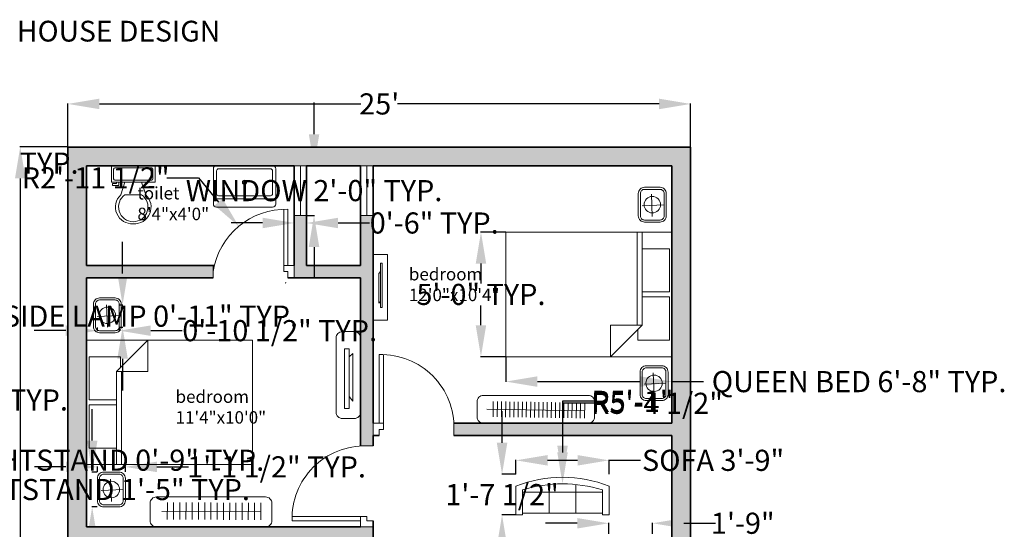
# Model space of a CAD drawing. Units: inches. Extents: x 19 to 15718, y 7 to 930.
# Tile 11 of 11: x 15243 to 15718, y 646 to 892. Entities that reach past the tile are written whole.
import ezdxf

# ---------------------------------------------------------------- set-up
doc = ezdxf.new("R2010")
doc.units = ezdxf.units.IN
doc.header["$MEASUREMENT"] = 0
for name, color, linetype, lineweight in [('A-ANNO-DIMS', 2, 'Continuous', 18), ('A-ANNO-TEXT', 7, 'Continuous', 25), ('A-AREA-IDEN', 7, 'Continuous', 18), ('A-DOOR', 4, 'Continuous', 20), ('A-FLOR-CASE', 8, 'Continuous', 18), ('A-FLOR-FIXT', 9, 'Continuous', 18), ('A-FURN', 8, 'Continuous', 18), ('A-GLAZ', 4, 'Continuous', 18), ('A-WALL', 7, 'Continuous', 35)]:
    doc.layers.add(name, color=color, linetype=linetype, lineweight=lineweight)
doc.layers.add('A-WALL-PATT', color=18, linetype='Continuous', lineweight=13, true_color=0x000000)
doc.styles.add('Annotative', font='arial.ttf')
doc.styles.get("Standard").update_dxf_attribs({"font": 'arial.ttf'})
doc.dimstyles.get("Standard").update_dxf_attribs({"dimtxt": 10.18, "dimasz": 15.18, "dimexe": 0.18, "dimexo": 0.0625, "dimgap": 0.09, "dimtad": 0, "dimtih": 1, "dimtoh": 1, "dimdec": 0, "dimzin": 0, "dimdsep": 46, "dimlunit": 3, "dimtxsty": 'Standard', "dimcen": 0.09, "dimadec": 0, "dimazin": 0, "dimtfac": 1, "dimtdec": 0, "dimtofl": 0, "dimtmove": 0, "dimatfit": 3, "dimfxl": 1, "dimtolj": 1, "dimtzin": 0, "dimarcsym": 0})

# ---------------------------------------------------------------- blocks, each defined once
blk = doc.blocks.new('Bed - Queen')
for p, q in [((0, -80.00003), (0, 0)), ((0, 0), (59.99999, 0)), ((59.99999, 0), (59.99999, -80.00003)), ((7.99999, -1.2), (28.79998, -1.2)), ((7.99999, -14.4), (7.99999, -1.2)), ((28.79998, -1.2), (28.79998, -14.4)), ((31.19999, -1.2), (51.99999, -1.2)), ((31.19999, -14.4), (31.19999, -1.2)), ((51.99999, -1.2), (51.99999, -16.4)), ((0, -14.4), (44.8, -14.4)), ((44.8, -16.8), (0, -16.8)), ((59.99999, -29.6), (44.8, -14.4)), ((44.8, -14.4), (44.8, -29.6)), ((51.99999, -16.4), (46.79936, -16.4)), ((44.8, -29.6), (59.99999, -29.6)), ((59.99999, -80.00003), (0, -80.00003))]:
    blk.add_line(p, q)
blk = doc.blocks.new('Sofa - Roundback 7 ft.')
for p, q in [((-12.00002, -32.4421), (-12.00003, -6.5971)), ((11.99997, -32.4421), (11.99998, -6.5971)), ((-36.000027, -34), (-36.000027, -11.4696)), ((-35.999844, -13.3819), (35.9998, -13.3819)), ((35.99998, -34), (35.99998, -11.4696)), ((-36.000027, -32.4421), (35.99998, -32.4421))]:
    blk.add_line(p, q)
for points in [[(-36.000027, -34), (-42.000027, -34), (-42.000027, -8)], [(41.99998, -8), (41.99998, -34), (35.99998, -34)]]:
    blk.add_lwpolyline(points)
for centre, radius, start, end in [((0, -114.25), 114.25, 68.43141, 111.5686), ((-0.00001, -127.1968), 121.1968, 72.72033, 107.2797)]:
    blk.add_arc(centre, radius, start, end)
blk = doc.blocks.new('*D16')
at = {"layer": 'A-ANNO-DIMS', "color": 0, "lineweight": -2, "transparency": 16777216}
for p, q in [((15266.68, 830.27), (15266.68, 851.13)), ((15281.86, 850.95), (15407.87, 850.95)), ((15551.5, 850.95), (15425.5, 850.95)), ((15566.68, 830.27), (15566.68, 851.13))]:
    blk.add_line(p, q, dxfattribs=at)
at = {"layer": 'A-ANNO-DIMS', "color": 0, "transparency": 16777216}
for points in [[(15281.86, 853.48), (15281.86, 848.42), (15266.68, 850.95)], [(15551.5, 853.48), (15551.5, 848.42), (15566.68, 850.95)]]:
    blk.add_solid(points, dxfattribs=at)
at = {"layer": 'Defpoints', "color": 0, "transparency": 16777216}
for p in [(15566.68, 850.95), (15266.68, 830.2), (15566.68, 830.2)]:
    blk.add_point(p, dxfattribs=at)
at = {"layer": 'A-ANNO-DIMS', "color": 0, "transparency": 16777216, "insert": (15416.68, 850.95), "char_height": 10.18, "attachment_point": 5}
blk.add_mtext("\\A1;25'", dxfattribs=at)
blk = doc.blocks.new('*D17')
at = {"layer": 'A-ANNO-DIMS', "color": 0, "lineweight": -2, "transparency": 16777216}
for p, q in [((15266.62, 830.27), (15243.58, 830.27)), ((15243.76, 815.09), (15243.76, 595.52)), ((15243.76, 365.38), (15243.76, 584.95)), ((15266.62, 350.2), (15243.58, 350.2))]:
    blk.add_line(p, q, dxfattribs=at)
at = {"layer": 'A-ANNO-DIMS', "color": 0, "transparency": 16777216}
for points in [[(15241.23, 815.09), (15246.29, 815.09), (15243.76, 830.27)], [(15241.23, 365.38), (15246.29, 365.38), (15243.76, 350.2)]]:
    blk.add_solid(points, dxfattribs=at)
at = {"layer": 'Defpoints', "color": 0, "transparency": 16777216}
for p in [(15266.68, 830.27), (15243.76, 350.2), (15266.68, 350.2)]:
    blk.add_point(p, dxfattribs=at)
at = {"layer": 'A-ANNO-DIMS', "color": 0, "transparency": 16777216, "insert": (15243.76, 590.24), "char_height": 10.18, "attachment_point": 5}
blk.add_mtext("\\A1;40'", dxfattribs=at)
blk = doc.blocks.new('*U2')
for p, q in [((9.5, -6), (9.5, -2)), ((-10, -8.5), (-8, -8.5)), ((-10, -9.5), (-10, -8.5)), ((-8, -8.5), (-8, -8)), ((-7, -8), (-7, -9.5)), ((-4, -8), (-6, -14)), ((4, -8), (6, -14)), ((-7, -9.5), (-10, -9.5)), ((4, -14), (-4, -14))]:
    blk.add_line(p, q)
blk.add_lwpolyline([(10.5, -8), (10.5, 0), (-10.5, 0), (-10.5, -8)], close=True)
for points in [[(-9.5, -2), (-9.5, -6)], [(8.5, -1), (-8.5, -1)], [(-8.5, -7), (8.5, -7)]]:
    blk.add_lwpolyline(points)
for centre, radius, start, end in [((-8.625, -1.875), 0.8839, 81.8699, 188.1301), ((8.625, -1.875), 0.8839, 351.8699, 98.1301), ((-8.625, -6.125), 0.8839, 171.869898, 278.1301), ((8.625, -6.125), 0.8839, 261.8699, 8.1301), ((-0.4772, -19.9188), 8.0953, 133.01722, 273.38), ((0.0374, -19.8731), 7.127, 124.50543, 269.7), ((-0.0373, -19.8731), 7.127, 270.3, 55.4946), ((0.4773, -19.9188), 8.0953, 266.62, 46.9828)]:
    blk.add_arc(centre, radius, start, end)
blk = doc.blocks.new('Sink-single - 30 in top')
blk.add_line((-15, -3.999996), (15, -3.999996))
for points in [[(-13.5, 0), (13.5, 0)], [(-15, -18.499996), (-15, -1.5)], [(15, -1.5), (15, -18.499996)], [(-13.5, -17.499996), (-13.5, -6.499996)], [(-12.5, -5.499996), (12.5, -5.499996)], [(13.5, -6.499996), (13.5, -17.499996)], [(12.5, -18.499996), (-12.5, -18.499996)], [(13.5, -19.999996), (-13.5, -19.999996)]]:
    blk.add_lwpolyline(points)
for radius in [1, 0.5]:
    blk.add_circle((0, -11.999996), radius)
for centre, radius, start, end in [((-13.5, -1.5), 1.5, 90, 180), ((13.5, -1.5), 1.5, 0, 90), ((-12.5, -6.499996), 1, 90, 180), ((12.5, -6.499996), 1, 0, 90), ((-13.5, -18.499996), 1.5, 180, 270), ((-12.5, -17.499996), 1, 180, 270), ((12.5, -17.499996), 1, 270, 0), ((13.5, -18.499996), 1.5, 270, 0)]:
    blk.add_arc(centre, radius, start, end)
blk = doc.blocks.new('DOOR-SWING-36IN')
for p, q in [((34.01, 3), (34.01, 39)), ((36.01, 6), (36.01, 39)), ((0.01, 6), (0.01, 0)), ((34.01, 6), (39.01, 6)), ((39.01, 6), (39.01, 0)), ((34.01, 3), (36.01, 3)), ((36.01, 3), (36.01, 0))]:
    blk.add_line(p, q)
blk.add_arc((35.01, 4), 35.01, 88.3634, 181.6366)
blk = doc.blocks.new('WIN-24IN-SINGLE-LINE')
for p, q in [((0, 24), (6, 24)), ((3, 24), (3, 0)), ((0, 0), (6, 0))]:
    blk.add_line(p, q)
blk = doc.blocks.new('NIGHTSTAND-LAMP')
for p, q in [((4.46, 10.77), (4.84, 0)), ((0, 5.25), (10.57, 5.76))]:
    blk.add_line(p, q)
blk.add_circle((4.84, 5.76), 3.96)
blk = doc.blocks.new('NIGHTSTAND-ROUNDED')
for points in [[(0, 13.79, -0.414214), (3, 16.79), (10.45, 16.79, -0.414214), (13.45, 13.79), (13.45, 3, -0.414214), (10.45, 0), (3, 0, -0.414214), (0, 3)], [(1, 13.79, -0.414214), (3, 15.79), (10.45, 15.79, -0.414214), (12.45, 13.79), (12.45, 3, -0.414214), (10.45, 1), (3, 1, -0.414214), (1, 3)]]:
    blk.add_lwpolyline(points, format="xyb", close=True)
blk = doc.blocks.new('*D38')
at = {"layer": 'A-ANNO-DIMS', "color": 0, "lineweight": -2, "transparency": 16777216}
for p, q in [((15293.05, 769.31), (15293.05, 784.49)), ((15291.5, 754.13), (15293.23, 754.13)), ((15291.5, 743.35), (15293.23, 743.35)), ((15293.05, 728.17), (15293.05, 712.99))]:
    blk.add_line(p, q, dxfattribs=at)
at = {"layer": 'A-ANNO-DIMS', "color": 0, "transparency": 16777216}
for points in [[(15290.52, 769.31), (15295.58, 769.31), (15293.05, 754.13)], [(15290.52, 728.17), (15295.58, 728.17), (15293.05, 743.35)]]:
    blk.add_solid(points, dxfattribs=at)
at = {"layer": 'Defpoints', "color": 0, "transparency": 16777216}
for p in [(15291.44, 754.13), (15293.05, 754.13), (15291.44, 743.35)]:
    blk.add_point(p, dxfattribs=at)
at = {"layer": 'A-ANNO-DIMS', "color": 0, "transparency": 16777216, "insert": (15293.05, 748.74), "char_height": 10.18, "attachment_point": 5}
blk.add_mtext('\\A1;BEDSIDE LAMP 0\'-11" TYP.', dxfattribs=at)
blk = doc.blocks.new('*D39')
at = {"layer": 'A-ANNO-DIMS', "color": 0, "lineweight": -2, "transparency": 16777216}
for p, q in [((15265.69, 741.74), (15250.51, 741.74)), ((15280.87, 743.29), (15280.87, 741.56)), ((15291.44, 743.29), (15291.44, 741.56)), ((15306.62, 741.74), (15321.8, 741.74))]:
    blk.add_line(p, q, dxfattribs=at)
at = {"layer": 'A-ANNO-DIMS', "color": 0, "transparency": 16777216}
for points in [[(15265.69, 744.27), (15265.69, 739.21), (15280.87, 741.74)], [(15306.62, 744.27), (15306.62, 739.21), (15291.44, 741.74)]]:
    blk.add_solid(points, dxfattribs=at)
at = {"layer": 'Defpoints', "color": 0, "transparency": 16777216}
for p in [(15280.87, 743.35), (15291.44, 743.35), (15291.44, 741.74)]:
    blk.add_point(p, dxfattribs=at)
at = {"layer": 'A-ANNO-DIMS', "color": 0, "transparency": 16777216, "insert": (15368.73, 741.74), "char_height": 10.18, "attachment_point": 5}
blk.add_mtext('\\A1;0\'-10 1/2" TYP.', dxfattribs=at)
blk = doc.blocks.new('*D44')
at = {"layer": 'A-ANNO-DIMS', "color": 0, "lineweight": -2, "transparency": 16777216}
for p, q in [((15477.68, 729.14), (15477.68, 717.02)), ((15557.68, 729.14), (15557.68, 717.02)), ((15492.86, 717.2), (15542.5, 717.2)), ((15557.68, 717.2), (15572.86, 717.2))]:
    blk.add_line(p, q, dxfattribs=at)
at = {"layer": 'A-ANNO-DIMS', "color": 0, "transparency": 16777216}
for points in [[(15492.86, 719.73), (15492.86, 714.67), (15477.68, 717.2)], [(15542.5, 719.73), (15542.5, 714.67), (15557.68, 717.2)]]:
    blk.add_solid(points, dxfattribs=at)
at = {"layer": 'Defpoints', "color": 0, "transparency": 16777216}
for p in [(15477.68, 729.2), (15557.68, 729.2), (15557.68, 717.2)]:
    blk.add_point(p, dxfattribs=at)
at = {"layer": 'A-ANNO-DIMS', "color": 0, "transparency": 16777216, "insert": (15647.82, 717.2), "char_height": 10.18, "attachment_point": 5}
blk.add_mtext('\\A1;QUEEN BED 6\'-8" TYP.', dxfattribs=at)
blk = doc.blocks.new('*D45')
at = {"layer": 'A-ANNO-DIMS', "color": 0, "lineweight": -2, "transparency": 16777216}
for p, q in [((15477.62, 789.2), (15465.5, 789.2)), ((15465.68, 774.02), (15465.68, 764.49)), ((15465.68, 744.38), (15465.68, 753.92)), ((15477.62, 729.2), (15465.5, 729.2))]:
    blk.add_line(p, q, dxfattribs=at)
at = {"layer": 'A-ANNO-DIMS', "color": 0, "transparency": 16777216}
for points in [[(15463.15, 774.02), (15468.21, 774.02), (15465.68, 789.2)], [(15463.15, 744.38), (15468.21, 744.38), (15465.68, 729.2)]]:
    blk.add_solid(points, dxfattribs=at)
at = {"layer": 'Defpoints', "color": 0, "transparency": 16777216}
for p in [(15477.68, 789.2), (15465.68, 729.2), (15477.68, 729.2)]:
    blk.add_point(p, dxfattribs=at)
at = {"layer": 'A-ANNO-DIMS', "color": 0, "transparency": 16777216, "insert": (15465.68, 759.2), "char_height": 10.18, "attachment_point": 5}
blk.add_mtext('\\A1;5\'-0" TYP.', dxfattribs=at)
blk = doc.blocks.new('*D48')
at = {"layer": 'A-ANNO-DIMS', "color": 0, "lineweight": -2, "transparency": 16777216}
for p, q in [((15076.85, 807.27), (15076.85, 822.45)), ((15076.85, 822.45), (15092.03, 822.45)), ((15081.77, 807.27), (15076.67, 807.27)), ((15076.85, 789.18), (15076.85, 792.09)), ((15081.77, 774), (15076.67, 774))]:
    blk.add_line(p, q, dxfattribs=at)
at = {"layer": 'A-ANNO-DIMS', "color": 0, "transparency": 16777216}
for points in [[(15074.32, 792.09), (15079.38, 792.09), (15076.85, 807.27)], [(15074.32, 789.18), (15079.38, 789.18), (15076.85, 774)]]:
    blk.add_solid(points, dxfattribs=at)
at = {"layer": 'Defpoints', "color": 0, "transparency": 16777216}
for p in [(15076.85, 807.27), (15081.84, 807.27), (15081.84, 774)]:
    blk.add_point(p, dxfattribs=at)
at = {"layer": 'A-ANNO-DIMS', "color": 0, "transparency": 16777216, "insert": (15184.13, 822.45), "char_height": 10.18, "attachment_point": 5}
blk.add_mtext('\\A1;DOOR SWING 2\'-9 1/2" TYP.', dxfattribs=at)
blk = doc.blocks.new('*D52')
at = {"layer": 'A-ANNO-DIMS', "color": 0, "lineweight": -2, "transparency": 16777216}
for p, q in [((15385.28, 836.38), (15385.28, 851.56)), ((15381.74, 821.2), (15385.46, 821.2)), ((15381.74, 797.2), (15385.46, 797.2)), ((15385.28, 782.02), (15385.28, 766.84))]:
    blk.add_line(p, q, dxfattribs=at)
at = {"layer": 'A-ANNO-DIMS', "color": 0, "transparency": 16777216}
for points in [[(15382.75, 836.38), (15387.81, 836.38), (15385.28, 821.2)], [(15382.75, 782.02), (15387.81, 782.02), (15385.28, 797.2)]]:
    blk.add_solid(points, dxfattribs=at)
at = {"layer": 'Defpoints', "color": 0, "transparency": 16777216}
for p in [(15381.68, 821.2), (15385.28, 821.2), (15381.68, 797.2)]:
    blk.add_point(p, dxfattribs=at)
at = {"layer": 'A-ANNO-DIMS', "color": 0, "transparency": 16777216, "insert": (15385.28, 809.2), "char_height": 10.18, "attachment_point": 5}
blk.add_mtext('\\A1;WINDOW 2\'-0" TYP.', dxfattribs=at)
blk = doc.blocks.new('*D53')
at = {"layer": 'A-ANNO-DIMS', "color": 0, "lineweight": -2, "transparency": 16777216}
for p, q in [((15375.68, 797.14), (15375.68, 793.42)), ((15381.68, 797.14), (15381.68, 793.42)), ((15360.5, 793.6), (15345.32, 793.6)), ((15396.86, 793.6), (15412.04, 793.6))]:
    blk.add_line(p, q, dxfattribs=at)
at = {"layer": 'A-ANNO-DIMS', "color": 0, "transparency": 16777216}
for points in [[(15360.5, 796.13), (15360.5, 791.07), (15375.68, 793.6)], [(15396.86, 796.13), (15396.86, 791.07), (15381.68, 793.6)]]:
    blk.add_solid(points, dxfattribs=at)
at = {"layer": 'Defpoints', "color": 0, "transparency": 16777216}
for p in [(15375.68, 797.2), (15381.68, 797.2), (15381.68, 793.6)]:
    blk.add_point(p, dxfattribs=at)
at = {"layer": 'A-ANNO-DIMS', "color": 0, "transparency": 16777216, "insert": (15443.16, 793.6), "char_height": 10.18, "attachment_point": 5}
blk.add_mtext('\\A1;0\'-6" TYP.', dxfattribs=at)
blk = doc.blocks.new('*D56')
at = {"layer": 'A-ANNO-DIMS', "color": 0, "lineweight": -2, "transparency": 16777216}
for p, q in [((15151.7, 679.35), (15136.52, 679.35)), ((15166.88, 678.06), (15166.88, 679.53)), ((15175.86, 678.06), (15175.86, 679.53)), ((15191.04, 679.35), (15206.22, 679.35))]:
    blk.add_line(p, q, dxfattribs=at)
at = {"layer": 'A-ANNO-DIMS', "color": 0, "transparency": 16777216}
for points in [[(15151.7, 681.88), (15151.7, 676.82), (15166.88, 679.35)], [(15191.04, 681.88), (15191.04, 676.82), (15175.86, 679.35)]]:
    blk.add_solid(points, dxfattribs=at)
at = {"layer": 'Defpoints', "color": 0, "transparency": 16777216}
for p in [(15175.86, 679.35), (15166.88, 678), (15175.86, 678)]:
    blk.add_point(p, dxfattribs=at)
at = {"layer": 'A-ANNO-DIMS', "color": 0, "transparency": 16777216, "insert": (15285.29, 679.35), "char_height": 10.18, "attachment_point": 5}
blk.add_mtext('\\A1;NIGHTSTAND 0\'-9" TYP.', dxfattribs=at)
blk = doc.blocks.new('*D57')
at = {"layer": 'A-ANNO-DIMS', "color": 0, "lineweight": -2, "transparency": 16777216}
for p, q in [((15165.53, 693.18), (15165.53, 708.36)), ((15165.53, 708.36), (15180.71, 708.36)), ((15166.82, 678), (15165.35, 678)), ((15166.82, 669.42), (15165.35, 669.42)), ((15165.53, 654.24), (15165.53, 639.06))]:
    blk.add_line(p, q, dxfattribs=at)
at = {"layer": 'A-ANNO-DIMS', "color": 0, "transparency": 16777216}
for points in [[(15163, 693.18), (15168.06, 693.18), (15165.53, 678)], [(15163, 654.24), (15168.06, 654.24), (15165.53, 669.42)]]:
    blk.add_solid(points, dxfattribs=at)
at = {"layer": 'Defpoints', "color": 0, "transparency": 16777216}
for p in [(15165.53, 678), (15166.88, 678), (15166.88, 669.42)]:
    blk.add_point(p, dxfattribs=at)
at = {"layer": 'A-ANNO-DIMS', "color": 0, "transparency": 16777216, "insert": (15223.69, 708.36), "char_height": 10.18, "attachment_point": 5}
blk.add_mtext('\\A1;0\'-8 1/2" TYP.', dxfattribs=at)
blk = doc.blocks.new('*D58')
at = {"layer": 'A-ANNO-DIMS', "color": 0, "lineweight": -2, "transparency": 16777216}
for p, q in [((15278.41, 688.79), (15278.41, 703.97)), ((15280.87, 673.61), (15278.23, 673.61)), ((15280.87, 656.82), (15278.23, 656.82)), ((15278.41, 641.64), (15278.41, 626.46))]:
    blk.add_line(p, q, dxfattribs=at)
at = {"layer": 'A-ANNO-DIMS', "color": 0, "transparency": 16777216}
for points in [[(15275.88, 688.79), (15280.94, 688.79), (15278.41, 673.61)], [(15275.88, 641.64), (15280.94, 641.64), (15278.41, 656.82)]]:
    blk.add_solid(points, dxfattribs=at)
at = {"layer": 'Defpoints', "color": 0, "transparency": 16777216}
for p in [(15278.41, 673.61), (15280.93, 673.61), (15280.93, 656.82)]:
    blk.add_point(p, dxfattribs=at)
at = {"layer": 'A-ANNO-DIMS', "color": 0, "transparency": 16777216, "insert": (15278.41, 665.21), "char_height": 10.18, "attachment_point": 5}
blk.add_mtext('\\A1;NIGHTSTAND 1\'-5" TYP.', dxfattribs=at)
blk = doc.blocks.new('*D59')
at = {"layer": 'A-ANNO-DIMS', "color": 0, "lineweight": -2, "transparency": 16777216}
for p, q in [((15265.75, 676.12), (15250.57, 676.12)), ((15280.93, 673.67), (15280.93, 676.3)), ((15294.38, 673.67), (15294.38, 676.3)), ((15309.56, 676.12), (15324.74, 676.12))]:
    blk.add_line(p, q, dxfattribs=at)
at = {"layer": 'A-ANNO-DIMS', "color": 0, "transparency": 16777216}
for points in [[(15265.75, 678.65), (15265.75, 673.59), (15280.93, 676.12)], [(15309.56, 678.65), (15309.56, 673.59), (15294.38, 676.12)]]:
    blk.add_solid(points, dxfattribs=at)
at = {"layer": 'Defpoints', "color": 0, "transparency": 16777216}
for p in [(15280.93, 673.61), (15294.38, 676.12), (15294.38, 673.61)]:
    blk.add_point(p, dxfattribs=at)
at = {"layer": 'A-ANNO-DIMS', "color": 0, "transparency": 16777216, "insert": (15367.23, 676.12), "char_height": 10.18, "attachment_point": 5}
blk.add_mtext('\\A1;1\'-1 1/2" TYP.', dxfattribs=at)
blk = doc.blocks.new('*D70')
at = {"layer": 'A-ANNO-DIMS', "color": 0, "lineweight": -2, "transparency": 16777216}
for p, q in [((15482.56, 672.62), (15482.56, 679.46)), ((15497.74, 679.28), (15512.2, 679.28)), ((15527.38, 672.62), (15527.38, 679.46)), ((15527.38, 679.28), (15542.56, 679.28))]:
    blk.add_line(p, q, dxfattribs=at)
at = {"layer": 'A-ANNO-DIMS', "color": 0, "transparency": 16777216}
for points in [[(15497.74, 681.81), (15497.74, 676.75), (15482.56, 679.28)], [(15512.2, 681.81), (15512.2, 676.75), (15527.38, 679.28)]]:
    blk.add_solid(points, dxfattribs=at)
at = {"layer": 'Defpoints', "color": 0, "transparency": 16777216}
for p in [(15527.38, 679.28), (15482.56, 672.56), (15527.38, 672.56)]:
    blk.add_point(p, dxfattribs=at)
at = {"layer": 'A-ANNO-DIMS', "color": 0, "transparency": 16777216, "insert": (15577.5, 679.28), "char_height": 10.18, "attachment_point": 5}
blk.add_mtext('\\A1;SOFA 3\'-9"', dxfattribs=at)
blk = doc.blocks.new('*D71')
at = {"layer": 'A-ANNO-DIMS', "color": 0, "lineweight": -2, "transparency": 16777216}
for p, q in [((15475.84, 687.74), (15475.84, 702.92)), ((15482.5, 672.56), (15475.66, 672.56)), ((15482.5, 652.99), (15475.66, 652.99)), ((15475.84, 637.81), (15475.84, 622.63))]:
    blk.add_line(p, q, dxfattribs=at)
at = {"layer": 'A-ANNO-DIMS', "color": 0, "transparency": 16777216}
for points in [[(15473.31, 687.74), (15478.37, 687.74), (15475.84, 672.56)], [(15473.31, 637.81), (15478.37, 637.81), (15475.84, 652.99)]]:
    blk.add_solid(points, dxfattribs=at)
at = {"layer": 'Defpoints', "color": 0, "transparency": 16777216}
for p in [(15475.84, 672.56), (15482.56, 672.56), (15482.56, 652.99)]:
    blk.add_point(p, dxfattribs=at)
at = {"layer": 'A-ANNO-DIMS', "color": 0, "transparency": 16777216, "insert": (15475.84, 662.77), "char_height": 10.18, "attachment_point": 5}
blk.add_mtext('\\A1;1\'-7 1/2"', dxfattribs=at)
blk = doc.blocks.new('*D73')
at = {"layer": 'A-ANNO-DIMS', "color": 0, "lineweight": -2, "transparency": 16777216}
for p, q in [((15512.03, 648.97), (15496.85, 648.97)), ((15527.21, 643.85), (15527.21, 649.15)), ((15548.3, 643.85), (15548.3, 649.15)), ((15563.48, 648.97), (15578.66, 648.97))]:
    blk.add_line(p, q, dxfattribs=at)
at = {"layer": 'A-ANNO-DIMS', "color": 0, "transparency": 16777216}
for points in [[(15512.03, 651.5), (15512.03, 646.44), (15527.21, 648.97)], [(15563.48, 651.5), (15563.48, 646.44), (15548.3, 648.97)]]:
    blk.add_solid(points, dxfattribs=at)
at = {"layer": 'Defpoints', "color": 0, "transparency": 16777216}
for p in [(15548.3, 648.97), (15527.21, 643.79), (15548.3, 643.79)]:
    blk.add_point(p, dxfattribs=at)
at = {"layer": 'A-ANNO-DIMS', "color": 0, "transparency": 16777216, "insert": (15591.8, 648.97), "char_height": 10.18, "attachment_point": 5}
blk.add_mtext('\\A1;1\'-9"', dxfattribs=at)
blk = doc.blocks.new('*D89')
at = {"layer": 'A-ANNO-DIMS', "color": 0, "lineweight": -2, "transparency": 16777216}
for p, q in [((15314.39, 815.33), (15329.57, 815.33)), ((15329.57, 815.33), (15339.29, 803.67)), ((15371.59, 764.8), (15371.77, 764.8)), ((15371.68, 764.71), (15371.68, 764.89))]:
    blk.add_line(p, q, dxfattribs=at)
at = {"layer": 'A-ANNO-DIMS', "color": 0, "transparency": 16777216}
blk.add_solid([(15341.23, 805.29), (15337.35, 802.05), (15349.01, 792.01)], dxfattribs=at)
at = {"layer": 'Defpoints', "color": 0, "transparency": 16777216}
for p in [(15349.01, 792.01), (15371.68, 764.8)]:
    blk.add_point(p, dxfattribs=at)
at = {"layer": 'A-ANNO-DIMS', "color": 0, "transparency": 16777216, "insert": (15280.09, 815.33), "char_height": 10.18, "attachment_point": 5}
blk.add_mtext('\\A1;R2\'-11 1/2"', dxfattribs=at)
blk = doc.blocks.new('*D90')
at = {"layer": 'A-ANNO-DIMS', "color": 0, "lineweight": -2, "transparency": 16777216}
for p, q in [((15520.15, 706.74), (15504.97, 706.74)), ((15504.97, 706.74), (15504.97, 683.11)), ((15504.88, 603.26), (15505.06, 603.26)), ((15504.97, 603.17), (15504.97, 603.35))]:
    blk.add_line(p, q, dxfattribs=at)
at = {"layer": 'A-ANNO-DIMS', "color": 0, "transparency": 16777216}
blk.add_solid([(15502.44, 683.11), (15507.5, 683.11), (15504.97, 667.93)], dxfattribs=at)
at = {"layer": 'Defpoints', "color": 0, "transparency": 16777216}
for p in [(15504.97, 667.93), (15504.97, 603.26)]:
    blk.add_point(p, dxfattribs=at)
at = {"layer": 'A-ANNO-DIMS', "color": 0, "transparency": 16777216, "insert": (15550.51, 706.74), "char_height": 10.18, "attachment_point": 5}
blk.add_mtext('\\A1;R5\'-4 1/2"', dxfattribs=at)
blk = doc.blocks.new('*D91')
at = {"layer": 'A-ANNO-DIMS', "color": 0, "lineweight": -2, "transparency": 16777216}
for p, q in [((15520.15, 707.71), (15504.97, 707.71)), ((15504.97, 707.71), (15504.97, 686.31)), ((15504.88, 610.17), (15505.06, 610.17)), ((15504.97, 610.08), (15504.97, 610.26))]:
    blk.add_line(p, q, dxfattribs=at)
at = {"layer": 'A-ANNO-DIMS', "color": 0, "transparency": 16777216}
blk.add_solid([(15502.44, 686.31), (15507.5, 686.31), (15504.97, 671.13)], dxfattribs=at)
at = {"layer": 'Defpoints', "color": 0, "transparency": 16777216}
for p in [(15504.97, 671.13), (15504.97, 610.17)]:
    blk.add_point(p, dxfattribs=at)
at = {"layer": 'A-ANNO-DIMS', "color": 0, "transparency": 16777216, "insert": (15538.64, 707.71), "char_height": 10.18, "attachment_point": 5}
blk.add_mtext('\\A1;R5\'-1"', dxfattribs=at)

msp = doc.modelspace()

# ---------------------------------------------------------------- hatches: boundary and pattern name
at = {"layer": 'A-WALL-PATT'}
h = msp.add_hatch(color=256, dxfattribs=at)
h.dxf.hatch_style = 1
h.paths.add_polyline_path([(15190.84, 837), (14890.84, 837), (14890.84, 357), (14899.84, 357), (14899.84, 366), (14899.84, 528), (14904.84, 528), (14904.84, 534), (14899.84, 534), (14899.84, 698), (15004.84, 698), (15004.84, 701, -0.014283), (15004.84, 703), (15004.84, 704), (14899.84, 704), (14899.84, 828), (14987.26, 828), (15043.84, 828), (15049.84, 828), (15075.84, 828), (15081.84, 828), (15181.84, 828), (15181.84, 780), (15114.84, 780), (15114.84, 779, -0.017236), (15114.84, 777), (15114.84, 774), (15181.84, 774), (15181.84, 654), (15181.84, 648), (15181.84, 596), (15190.84, 596)])
h.paths.add_polyline_path([(15190.84, 590), (15181.84, 590), (15181.84, 470), (15181.84, 464), (15181.84, 361.43), (14991.9, 361.43), (14991.5, 357), (15190.84, 357)], flags=0)
h.paths.add_polyline_path([(15152.29, 608), (15146.29, 608), (15146.29, 596), (15049.84, 596), (15049.84, 590), (15152.29, 590)], flags=17)
h.paths.add_polyline_path([(15049.84, 615), (15048.84, 615, -0.017236), (15046.84, 615), (15043.84, 615), (15043.84, 596), (15049.84, 596)], flags=17)
edge = h.paths.add_edge_path(flags=17)
edge.add_line((15152.29, 654), (15049.84, 654))
edge.add_line((15049.84, 654), (15043.84, 654))
edge.add_line((15043.84, 654), (15043.84, 648))
edge.add_line((15043.84, 648), (15049.84, 648))
edge.add_line((15049.84, 648), (15075.84, 648))
edge.add_line((15075.84, 648), (15081.84, 648))
edge.add_line((15081.84, 648), (15117.26, 648))
edge.add_spline(control_points=[(15117.26, 648), (15117.59, 648.02), (15117.94, 648.03), (15118.71, 648.04), (15119.15, 648.02), (15119.59, 648)], knot_values=[1.499122, 1.499122, 1.499122, 1.499122, 1.618335, 1.618335, 1.770388, 1.770388, 1.770388, 1.770388], degree=3, periodic=0)
edge.add_spline(control_points=[(15127.99, 642.93), (15128, 643.28), (15127.95, 643.62), (15127.73, 644.26), (15127.57, 644.57), (15127.16, 645.13), (15126.92, 645.39), (15126.04, 646.16), (15125.28, 646.6), (15123.53, 647.31), (15122.55, 647.59), (15120.88, 647.88), (15120.24, 647.95), (15119.59, 648)], knot_values=[0, 0, 0, 0, 0.172075, 0.172075, 0.344149, 0.344149, 0.516224, 0.516224, 0.894541, 0.894541, 1.272858, 1.272858, 1.499122, 1.499122, 1.499122, 1.499122], degree=3, periodic=0)
edge.add_line((15119.59, 648), (15146.29, 648))
edge.add_line((15146.29, 648), (15146.29, 636))
edge.add_line((15146.29, 636), (15152.29, 636))
edge.add_line((15152.29, 636), (15152.29, 654))
h.paths.add_polyline_path([(15132.35, 430.4), (15123.35, 430.4), (15123.35, 396.8), (15027.77, 396.8), (15027.77, 387.8), (15132.35, 387.8)], flags=17)
h.paths.add_polyline_path([(15132.35, 464), (15123.35, 464), (15123.35, 430.4), (15132.35, 430.4)], flags=17)
h.paths.add_polyline_path([(15275.68, 583.59), (15276.07, 583.2), (15276.65, 583.2), (15280.6, 587.16), (15278.55, 589.2), (15275.68, 589.2), (15275.68, 601.2), (15266.68, 601.2), (15266.68, 350.2), (15275.68, 350.2), (15275.68, 359.2), (15275.68, 457.2), (15413.68, 457.2), (15413.68, 471.04), (15407.68, 471.04), (15407.68, 463.2), (15275.68, 463.2)])
h = msp.add_hatch(color=256, dxfattribs=at)
h.dxf.hatch_style = 1
h.paths.add_polyline_path([(15566.68, 830.2), (15266.68, 830.2), (15266.68, 629.2), (15275.68, 629.2), (15275.68, 641.2), (15301.68, 641.2), (15301.68, 589.2), (15275.68, 589.2), (15275.68, 601.2), (15266.68, 601.2), (15266.68, 350.2), (15275.68, 350.2), (15275.68, 359.2), (15275.68, 457.2), (15413.68, 457.2), (15413.68, 471.04), (15407.68, 471.04), (15407.68, 463.2), (15275.68, 463.2), (15275.68, 583.59), (15276.07, 583.2), (15276.65, 583.2), (15277.42, 583.97), (15276.36, 585.03), (15279.54, 588.22), (15280.6, 587.16), (15281.66, 588.22), (15282.72, 587.16), (15283.78, 588.22), (15284.85, 587.16), (15285.91, 588.22), (15286.97, 587.16), (15288.03, 588.22), (15289.09, 587.16), (15290.15, 588.22), (15291.21, 587.16), (15292.27, 588.22), (15293.33, 587.16), (15294.39, 588.22), (15295.45, 587.16), (15296.51, 588.22), (15297.57, 587.16), (15298.63, 588.22), (15299.69, 587.16), (15300.76, 588.22), (15301.82, 587.16), (15302.88, 588.22), (15303.94, 587.16), (15305, 588.22), (15306.06, 587.16), (15307.68, 588.78), (15307.68, 641.2), (15407.68, 641.2), (15413.68, 641.2), (15413.68, 647.2), (15407.68, 647.2), (15275.68, 647.2), (15275.68, 767.2), (15336.68, 767.2), (15336.68, 773.2), (15275.68, 773.2), (15275.68, 821.2), (15375.68, 821.2), (15381.68, 821.2), (15407.68, 821.2), (15413.68, 821.2), (15557.68, 821.2), (15557.68, 697.2), (15452.68, 697.2), (15452.68, 696.2, -0.014283), (15452.68, 694.2), (15452.68, 691.2), (15557.68, 691.2), (15557.68, 527.2), (15557.68, 521.2), (15557.68, 359.2), (15557.68, 350.2), (15566.68, 350.2)])
h.paths.add_polyline_path([(15416.63, 527.2), (15413.68, 527.2), (15407.68, 527.2), (15407.68, 521.04), (15413.68, 521.04), (15413.68, 521.2), (15416.63, 521.2)], flags=17)
h.paths.add_polyline_path([(15432.13, 393.97), (15308.13, 393.97), (15308.13, 425.59), (15299.13, 425.59), (15299.13, 384.97), (15432.13, 384.97)], flags=17)
h.paths.add_polyline_path([(15308.13, 457.2), (15299.13, 457.2), (15299.13, 425.59), (15308.13, 425.59)], flags=17)
h.paths.add_polyline_path([(15425.57, 359.2), (15275.68, 359.2), (15275.68, 350.2), (15425.57, 350.2)], flags=17)
h.paths.add_polyline_path([(15413.68, 797.2), (15407.68, 797.2), (15407.68, 773.2), (15381.68, 773.2), (15381.68, 797.2), (15375.68, 797.2), (15375.68, 773.2), (15375.68, 767.2), (15407.68, 767.2), (15407.68, 686.2), (15408.68, 686.2, -0.014283), (15410.68, 686.2), (15413.68, 686.2), (15413.68, 691.2), (15413.68, 697.2)], flags=17)
h.paths.add_polyline_path([(15413.68, 608.2), (15410.68, 608.2, -0.017236), (15408.68, 608.2), (15407.68, 608.2), (15407.68, 589.2), (15388.16, 589.2, -0.313626), (15386.75, 588.23), (15381.37, 588.23), (15380.3, 587.16), (15381.37, 586.1), (15380.3, 585.03), (15382.14, 583.2), (15407.68, 583.2), (15413.68, 583.2)], flags=17)

# ---------------------------------------------------------------- linework, layer by layer
at = {"layer": 'A-DOOR'}
for p, q in [((15370.68, 770.2), (15370.68, 800.2)), ((15372.68, 773.2), (15372.68, 800.2)), ((15336.68, 773.2), (15336.68, 767.2)), ((15370.68, 773.2), (15375.68, 773.2)), ((15375.68, 773.2), (15375.68, 767.2)), ((15370.68, 770.2), (15372.68, 770.2)), ((15372.68, 770.2), (15372.68, 767.2))]:
    msp.add_line(p, q, dxfattribs=at)
msp.add_arc((15371.68, 764.8), 35.41, 88.3819, 171.2292, dxfattribs=at)
at = {"layer": 'A-FLOR-CASE'}
for p, q in [((15471.64, 707.64), (15471.54, 700.23)), ((15473.64, 707.61), (15473.54, 700.21)), ((15475.64, 707.58), (15475.54, 700.18)), ((15477.64, 707.55), (15477.54, 700.15)), ((15479.64, 707.52), (15479.54, 700.12)), ((15481.64, 707.49), (15481.54, 700.09)), ((15483.64, 707.46), (15483.53, 700.06)), ((15485.64, 707.43), (15485.53, 700.03)), ((15487.64, 707.4), (15487.53, 700)), ((15489.64, 707.38), (15489.53, 699.97)), ((15491.64, 707.35), (15491.53, 699.94)), ((15493.64, 707.32), (15493.53, 699.91)), ((15495.64, 707.29), (15495.53, 699.88)), ((15497.64, 707.26), (15497.53, 699.85)), ((15499.64, 707.23), (15499.53, 699.82)), ((15501.64, 707.2), (15501.53, 699.8)), ((15503.64, 707.17), (15503.53, 699.77)), ((15505.64, 707.14), (15505.53, 699.74)), ((15507.64, 707.11), (15507.53, 699.71)), ((15509.64, 707.08), (15509.53, 699.68)), ((15511.64, 707.05), (15511.53, 699.65)), ((15513.64, 707.02), (15513.53, 699.62)), ((15515.64, 706.99), (15515.53, 699.59)), ((15468.54, 703.85), (15515.6, 703.16)), ((15311.91, 654.63), (15359.5, 654.43)), ((15314.64, 658.98), (15314.6, 650.8)), ((15317.64, 658.96), (15317.6, 650.79)), ((15320.64, 658.95), (15320.6, 650.78)), ((15323.64, 658.94), (15323.6, 650.76)), ((15326.64, 658.93), (15326.6, 650.75)), ((15329.64, 658.91), (15329.6, 650.74)), ((15332.64, 658.9), (15332.6, 650.72)), ((15335.64, 658.89), (15335.6, 650.71)), ((15338.64, 658.87), (15338.6, 650.7)), ((15341.64, 658.86), (15341.6, 650.68)), ((15344.64, 658.85), (15344.6, 650.67)), ((15347.64, 658.83), (15347.6, 650.66)), ((15350.64, 658.82), (15350.6, 650.64)), ((15353.64, 658.81), (15353.6, 650.63)), ((15356.64, 658.79), (15356.6, 650.62)), ((15359.64, 658.78), (15359.6, 650.6))]:
    msp.add_line(p, q, dxfattribs=at)
for points in [[(15463.78, 700.2, 0.414214), (15466.78, 697.2), (15517.44, 697.2, 0.414214), (15520.44, 700.2), (15520.44, 707.51, 0.414214), (15517.44, 710.51), (15466.78, 710.51, 0.414214), (15463.78, 707.51)], [(15306.35, 650.2, 0.414214), (15309.35, 647.2), (15361.94, 647.2, 0.414214), (15364.94, 650.2), (15364.94, 658.65, 0.414214), (15361.94, 661.65), (15309.35, 661.65, 0.414214), (15306.35, 658.65)]]:
    msp.add_lwpolyline(points, format="xyb", close=True, dxfattribs=at)
at = {"layer": 'A-FURN'}
for p, q in [((15416.53, 769.26), (15416.51, 754.93)), ((15417.25, 770.25), (15416.53, 769.26)), ((15417.25, 771.72), (15417.25, 770.25)), ((15416.51, 754.93), (15417.25, 755.76)), ((15402.12, 729.1), (15403.99, 730.69)), ((15403.99, 730.69), (15403.99, 707.73)), ((15403.99, 707.73), (15402.12, 709.98))]:
    msp.add_line(p, q, dxfattribs=at)
for points in [[(15541.49, 807.81, -0.414214), (15544.49, 810.81), (15551.94, 810.81, -0.414214), (15554.94, 807.81), (15554.94, 797.02, -0.414214), (15551.94, 794.02), (15544.49, 794.02, -0.414214), (15541.49, 797.02)], [(15542.49, 807.81, -0.414214), (15544.49, 809.81), (15551.94, 809.81, -0.414214), (15553.94, 807.81), (15553.94, 797.02, -0.414214), (15551.94, 795.02), (15544.49, 795.02, -0.414214), (15542.49, 797.02)], [(15278.99, 754.51, -0.414214), (15281.99, 757.51), (15289.44, 757.51, -0.414214), (15292.44, 754.51), (15292.44, 743.72, -0.414214), (15289.44, 740.72), (15281.99, 740.72, -0.414214), (15278.99, 743.72)], [(15279.99, 754.51, -0.414214), (15281.99, 756.51), (15289.44, 756.51, -0.414214), (15291.44, 754.51), (15291.44, 743.72, -0.414214), (15289.44, 741.72), (15281.99, 741.72, -0.414214), (15279.99, 743.72)], [(15407.68, 738.27, 0.414214), (15404.68, 741.27), (15398.87, 741.27, 0.414214), (15395.87, 738.27), (15395.87, 702.45, 0.414214), (15398.87, 699.45), (15404.68, 699.45, 0.414214), (15407.68, 702.45)]]:
    msp.add_lwpolyline(points, format="xyb", close=True, dxfattribs=at)
for points in [[(15413.68, 778.38), (15413.68, 778.38), (15420.66, 778.38), (15420.66, 778.38), (15420.66, 746.81), (15420.66, 746.81), (15413.68, 746.81), (15413.68, 746.81)], [(15418.16, 774.22), (15418.16, 774.22), (15417.25, 774.22), (15417.25, 774.22), (15417.25, 752.9), (15417.25, 752.9), (15418.16, 752.9), (15418.16, 752.9)], [(15399.99, 732.95), (15399.99, 732.95), (15402.12, 732.95), (15402.12, 732.95), (15402.12, 704.28), (15402.12, 704.28), (15399.99, 704.28), (15399.99, 704.28)]]:
    msp.add_lwpolyline(points, close=True, dxfattribs=at)
at = {"layer": 'A-WALL'}
for p, q in [((15266.68, 350.2), (15266.68, 830.2)), ((15266.68, 830.2), (15566.68, 830.2)), ((15566.68, 830.2), (15566.68, 350.2)), ((15275.68, 821.2), (15375.68, 821.2)), ((15275.68, 773.2), (15275.68, 821.2)), ((15375.68, 773.2), (15375.68, 821.2)), ((15381.68, 773.2), (15381.68, 821.2)), ((15381.68, 821.2), (15407.68, 821.2)), ((15407.68, 821.2), (15407.68, 773.2)), ((15413.68, 821.2), (15413.68, 697.2)), ((15413.68, 821.2), (15557.68, 821.2)), ((15557.68, 821.2), (15557.68, 697.2)), ((15275.68, 773.2), (15337.28, 773.2)), ((15381.68, 773.2), (15407.68, 773.2)), ((15275.68, 767.2), (15336.68, 767.2)), ((15275.68, 647.2), (15275.68, 767.2)), ((15372.68, 767.2), (15407.68, 767.2)), ((15407.68, 767.2), (15407.68, 686.16)), ((15452.64, 697.2), (15557.68, 697.2)), ((15413.68, 691.2), (15416.68, 691.2)), ((15413.68, 691.2), (15413.68, 686.2)), ((15452.68, 691.2), (15557.68, 691.2)), ((15557.68, 691.2), (15557.68, 527.2)), ((15413.68, 650.2), (15413.68, 638.2)), ((15275.68, 647.2), (15407.68, 647.2))]:
    msp.add_line(p, q, dxfattribs=at)

# ---------------------------------------------------------------- block references
at = {"layer": 'A-DOOR', "extrusion": (0, 0, -1), "zscale": -1}
msp.add_blockref('DOOR-SWING-36IN', (-15452.69, 691.2), dxfattribs=at)
at = {"layer": 'A-DOOR', "extrusion": (0, 0, -1), "zscale": -1, "rotation": 269.9999999999739}
msp.add_blockref('DOOR-SWING-36IN', (-15413.68, 686.21), dxfattribs=at)
at = {"layer": 'A-FLOR-FIXT'}
msp.add_blockref('*U2', (15298.2, 821.2), dxfattribs=at)
at = {"layer": 'A-FLOR-FIXT', "rotation": 180}
msp.add_blockref('Sink-single - 30 in top', (15351.81, 801.2), dxfattribs=at)
at = {"layer": 'A-FURN'}
for name, p in [('NIGHTSTAND-LAMP', (15543.37, 796.65)), ('NIGHTSTAND-LAMP', (15280.87, 743.36)), ('NIGHTSTAND-ROUNDED', (15542.36, 708.02)), ('NIGHTSTAND-LAMP', (15544.24, 710.65)), ('NIGHTSTAND-ROUNDED', (15280.93, 656.82)), ('NIGHTSTAND-LAMP', (15282.81, 659.45))]:
    msp.add_blockref(name, p, dxfattribs=at)
for p, rotation in [((15557.68, 789.2), 270), ((15275.68, 677.2), 90)]:
    msp.add_blockref('Bed - Queen', p, dxfattribs=dict(at, rotation=rotation))
at = {"layer": 'A-FURN', "xscale": 0.5336144788434671, "yscale": 0.5336144788434671, "zscale": 0.5336144788434671}
msp.add_blockref('Sofa - Roundback 7 ft.', (15504.97, 671.13), dxfattribs=at)
at = {"layer": 'A-GLAZ'}
for p in [(15375.68, 797.2), (15407.68, 797.2)]:
    msp.add_blockref('WIN-24IN-SINGLE-LINE', p, dxfattribs=at)

# ---------------------------------------------------------------- texts
at = {"layer": 'A-ANNO-TEXT', "insert": (15107.17, 891), "char_height": 10, "attachment_point": 1}
msp.add_mtext_dynamic_manual_height_columns("25'x40' AFFORDABLE HOUSE DESIGN", width=556.6952, gutter_width=1, heights=[0], dxfattribs=at)
at = {"layer": 'A-AREA-IDEN', "char_height": 6, "width": 68.1983, "attachment_point": 1, "style": 'Annotative'}
for s, insert in [('toilet\\P8\'4"x4\'0"', (15300.19, 810.95)), ('bedroom\\P12\'0"x10\'4"', (15430.97, 771.96)), ('bedroom\\P11\'4"x10\'0"', (15318.58, 712.96))]:
    msp.add_mtext(s, dxfattribs=dict(at, insert=insert))

# ---------------------------------------------------------------- dimensions: what is measured, and where the dimension line sits
at = {"layer": 'A-ANNO-DIMS'}
for base, p1, p2, angle, text, picture, middle in [((15076.85, 807.27), (15081.84, 774), (15081.84, 807.27), 90, 'DOOR SWING <> TYP.', '*D48', (15184.13, 822.45)), ((15385.28, 821.2), (15381.68, 797.2), (15381.68, 821.2), 90, 'WINDOW <> TYP.', '*D52', (15385.28, 809.2)), ((15465.68, 729.2), (15477.68, 789.2), (15477.68, 729.2), 270, '<> TYP.', '*D45', (15465.68, 759.2)), ((15293.05, 754.13), (15291.44, 743.35), (15291.44, 754.13), 90, 'BEDSIDE LAMP <> TYP.', '*D38', (15293.05, 748.74)), ((15165.53, 678), (15166.88, 669.42), (15166.88, 678), 90, '<> TYP.', '*D57', (15223.69, 708.36)), ((15278.41, 673.61), (15280.93, 656.82), (15280.93, 673.61), 90, 'NIGHTSTAND <> TYP.', '*D58', (15278.41, 665.21))]:
    dim = msp.add_linear_dim(base=base, p1=p1, p2=p2, angle=angle, text=text, dimstyle='Standard', override={"dimdec": 1, "dimlfac": 1, "dimrnd": 0, "dimzin": 1, "dimdsep": 46, "dimlunit": 4, "dimfrac": 2}, dxfattribs=at)
    dim.commit()
    dim.dimension.update_dxf_attribs({"geometry": picture, "text_midpoint": middle})
for base, p1, p2, override, picture, middle in [((15566.68, 850.95), (15266.68, 830.2), (15566.68, 830.2), {"dimclrd": 0, "dimclre": 0, "dimclrt": 0}, '*D16', (15416.68, 850.95)), ((15548.3, 648.97), (15527.21, 643.79), (15548.3, 643.79), {"dimdec": 1, "dimlfac": 1, "dimrnd": 0, "dimzin": 1, "dimdsep": 46, "dimlunit": 4, "dimfrac": 2}, '*D73', (15591.8, 648.97))]:
    dim = msp.add_linear_dim(base=base, p1=p1, p2=p2, dimstyle='Standard', override=override, dxfattribs=at)
    dim.commit()
    dim.dimension.update_dxf_attribs({"geometry": picture, "text_midpoint": middle})
for base, p1, p2, override, picture, middle in [((15243.76, 350.2), (15266.68, 830.27), (15266.68, 350.2), {"dimclrd": 0, "dimclre": 0, "dimclrt": 0}, '*D17', (15243.76, 590.24)), ((15475.84, 672.56), (15482.56, 652.99), (15482.56, 672.56), {"dimdec": 1, "dimlfac": 1, "dimrnd": 0, "dimzin": 1, "dimdsep": 46, "dimlunit": 4, "dimfrac": 2}, '*D71', (15475.84, 662.77))]:
    dim = msp.add_linear_dim(base=base, p1=p1, p2=p2, angle=90, dimstyle='Standard', override=override, dxfattribs=at)
    dim.commit()
    dim.dimension.update_dxf_attribs({"geometry": picture, "text_midpoint": middle})
dim = msp.add_radius_dim(center=(15371.68, 764.8), mpoint=(15349.01, 792.01), dimstyle='Standard', override={"dimdec": 1, "dimlfac": 1, "dimrnd": 0, "dimzin": 1, "dimdsep": 46, "dimlunit": 4, "dimfrac": 2}, dxfattribs=at)
dim.commit()
dim.dimension.update_dxf_attribs({"geometry": '*D89', "text_midpoint": (15280.09, 815.33)})
for base, p1, p2, text, picture, middle in [((15381.68, 793.6), (15375.68, 797.2), (15381.68, 797.2), '<> TYP.', '*D53', (15443.16, 793.6)), ((15291.44, 741.74), (15280.87, 743.35), (15291.44, 743.35), '<> TYP.', '*D39', (15368.73, 741.74)), ((15557.68, 717.2), (15477.68, 729.2), (15557.68, 729.2), 'QUEEN BED <> TYP.', '*D44', (15647.82, 717.2)), ((15175.86, 679.35), (15166.88, 678), (15175.86, 678), 'NIGHTSTAND <> TYP.', '*D56', (15285.29, 679.35)), ((15294.3754, 676.124), (15280.93, 673.6062), (15294.3754, 673.6062), '<> TYP.', '*D59', (15367.2328, 676.124)), ((15527.38, 679.28), (15482.56, 672.56), (15527.38, 672.56), 'SOFA <>', '*D70', (15577.5, 679.28))]:
    dim = msp.add_linear_dim(base=base, p1=p1, p2=p2, text=text, dimstyle='Standard', override={"dimdec": 1, "dimlfac": 1, "dimrnd": 0, "dimzin": 1, "dimdsep": 46, "dimlunit": 4, "dimfrac": 2}, dxfattribs=at)
    dim.commit()
    dim.dimension.update_dxf_attribs({"geometry": picture, "text_midpoint": middle})
for center, mpoint, picture, middle in [((15504.97, 603.26), (15504.97, 667.93), '*D90', (15550.51, 706.74)), ((15504.97, 610.17), (15504.97, 671.13), '*D91', (15538.64, 707.71))]:
    dim = msp.add_radius_dim(center=center, mpoint=mpoint, dimstyle='Standard', override={"dimdec": 1, "dimlfac": 1, "dimrnd": 0, "dimzin": 1, "dimdsep": 46, "dimlunit": 4, "dimfrac": 2}, dxfattribs=at)
    dim.commit()
    dim.dimension.update_dxf_attribs({"geometry": picture, "text_midpoint": middle, "dimtype": 164})

doc.saveas('drawing.dxf')
